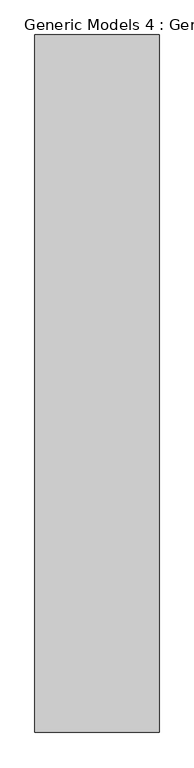
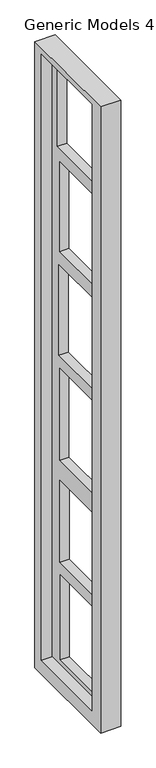
"""IFC4 building model written with IfcOpenShell, lengths in millimetres: proxy geometry, Generic Models 4 : Generic Models 1."""

from ifc_helpers import new_model, si_unit, origin, place, context, project, spatial, faceted_brep, source, transform, mapped, element, save


def generic_models_4_generic_models_1_30fca322(model_context):
    return source(origin(), model_context, "Body", "Brep", [
        faceted_brep([(-6457.5487703, -732.3037749, 18288.0), (-6457.5487703, 2442.6962251, 18288.0), (-7022.5256993, 2442.6962251, 18288.0), (-7022.5256993, -732.3037749, 18288.0), (-6457.5487703, -732.3037749, -158.4213758), (-7022.5256993, -732.3037749, -158.4213758), (-7022.5256993, 2442.6962251, -158.4213758), (-6457.5487703, 2442.6962251, -158.4213758), (-6457.5487703, 80.4962251, 15427.4465317), (-6457.5487703, 80.4962251, 17896.0910797), (-6457.5487703, 1889.1429371, 17896.0910797), (-6457.5487703, 1889.1429371, 15427.4465317), (-6457.5487703, -8.6872134, 12397.0580072), (-6457.5487703, -8.6872134, 15042.3231805), (-6457.5487703, 1781.5076359, 15042.3231805), (-6457.5487703, 1781.5076359, 12397.0580072), (-6457.5487703, -17.3853235, 9328.6434489), (-6457.5487703, -17.3853235, 11990.9234937), (-6457.5487703, 1807.8390259, 11990.9234937), (-6457.5487703, 1807.8390259, 9328.6434489), (-6457.5487703, -30.6801441, 6248.4), (-6457.5487703, -30.6801441, 8955.1024994), (-6457.5487703, 1778.1125113, 8955.1024994), (-6457.5487703, 1778.1125113, 6248.4), (-6457.5487703, -22.1772395, 3249.0844472), (-6457.5487703, -22.1772395, 5661.4894523), (-6457.5487703, 1769.7396662, 5661.4894523), (-6457.5487703, 1769.7396662, 3249.0844472), (-6457.5487703, -35.8456262, 382.1575328), (-6457.5487703, -35.8456262, 2893.6398867), (-6457.5487703, 1759.3912226, 2893.6398867), (-6457.5487703, 1759.3912226, 382.1575328), (-7022.5256993, -312.6392341, 18107.7487565), (-7022.5256993, -312.6392341, 247.1582995), (-7022.5256993, 2136.1756814, 247.1582995), (-7022.5256993, 2136.1756814, 18107.7487565), (-6717.7256993, -312.6392341, 18107.7487565), (-6717.7256993, 2136.1756814, 18107.7487565), (-6717.7256993, 2136.1756814, 247.1582995), (-6717.7256993, -312.6392341, 247.1582995), (-6717.7256993, 80.4962251, 17896.0910797), (-6717.7256993, 80.4962251, 15427.4465317), (-6717.7256993, 1889.1429371, 15427.4465317), (-6717.7256993, 1889.1429371, 17896.0910797), (-6717.7256993, -8.6872134, 15042.3231805), (-6717.7256993, -8.6872134, 12397.0580072), (-6717.7256993, 1781.5076359, 12397.0580072), (-6717.7256993, 1781.5076359, 15042.3231805), (-6717.7256993, -17.3853235, 11990.9234937), (-6717.7256993, -17.3853235, 9328.6434489), (-6717.7256993, 1807.8390259, 9328.6434489), (-6717.7256993, 1807.8390259, 11990.9234937), (-6717.7256993, -30.6801441, 8955.1024994), (-6717.7256993, -30.6801441, 6248.4), (-6717.7256993, 1778.1125113, 6248.4), (-6717.7256993, 1778.1125113, 8955.1024994), (-6717.7256993, -22.1772395, 5661.4894523), (-6717.7256993, -22.1772395, 3249.0844472), (-6717.7256993, 1769.7396662, 3249.0844472), (-6717.7256993, 1769.7396662, 5661.4894523), (-6717.7256993, -35.8456262, 2893.6398867), (-6717.7256993, -35.8456262, 382.1575328), (-6717.7256993, 1759.3912226, 382.1575328), (-6717.7256993, 1759.3912226, 2893.6398867)], [[[0, 1, 2, 3]], [[4, 5, 6, 7]], [[1, 0, 4, 7], [8, 9, 10, 11], [12, 13, 14, 15], [16, 17, 18, 19], [20, 21, 22, 23], [24, 25, 26, 27], [28, 29, 30, 31]], [[2, 1, 7, 6]], [[3, 2, 6, 5], [32, 33, 34, 35]], [[0, 3, 5, 4]], [[36, 37, 38, 39], [40, 41, 42, 43], [44, 45, 46, 47], [48, 49, 50, 51], [52, 53, 54, 55], [56, 57, 58, 59], [60, 61, 62, 63]], [[36, 39, 33, 32]], [[39, 38, 34, 33]], [[38, 37, 35, 34]], [[37, 36, 32, 35]], [[40, 9, 8, 41]], [[41, 8, 11, 42]], [[42, 11, 10, 43]], [[9, 40, 43, 10]], [[44, 13, 12, 45]], [[45, 12, 15, 46]], [[46, 15, 14, 47]], [[13, 44, 47, 14]], [[48, 17, 16, 49]], [[49, 16, 19, 50]], [[50, 19, 18, 51]], [[17, 48, 51, 18]], [[52, 21, 20, 53]], [[53, 20, 23, 54]], [[54, 23, 22, 55]], [[21, 52, 55, 22]], [[56, 25, 24, 57]], [[57, 24, 27, 58]], [[58, 27, 26, 59]], [[25, 56, 59, 26]], [[60, 29, 28, 61]], [[61, 28, 31, 62]], [[62, 31, 30, 63]], [[29, 60, 63, 30]]]),
    ])


if __name__ == "__main__":
    model = new_model("IFC4")
    model_context = context("Model", 3, world=origin())
    ifc_project = project(units=[si_unit("LENGTHUNIT", "METRE", prefix="MILLI")], contexts=[model_context])
    site = spatial("IfcSite", under=ifc_project)
    building = spatial("IfcBuilding", under=site)
    placement = place(None, origin())
    generic_models_4_generic_models_1_shape = generic_models_4_generic_models_1_30fca322(model_context)
    element("IfcBuildingElementProxy", 1, Name="Generic Models 4 : Generic Models 1", ObjectType="Generic Models 4 : Generic Models 1", at=placement, inside=building, context=model_context, shape_type="MappedRepresentation", body=[
        mapped(generic_models_4_generic_models_1_shape, transform((0.0, 0.0, 0.0), x_axis=(1.0, 0.0, 0.0), y_axis=(0.0, 1.0, 0.0), z_axis=(0.0, 0.0, 1.0))),
    ])
    save(model, "model.ifc")
